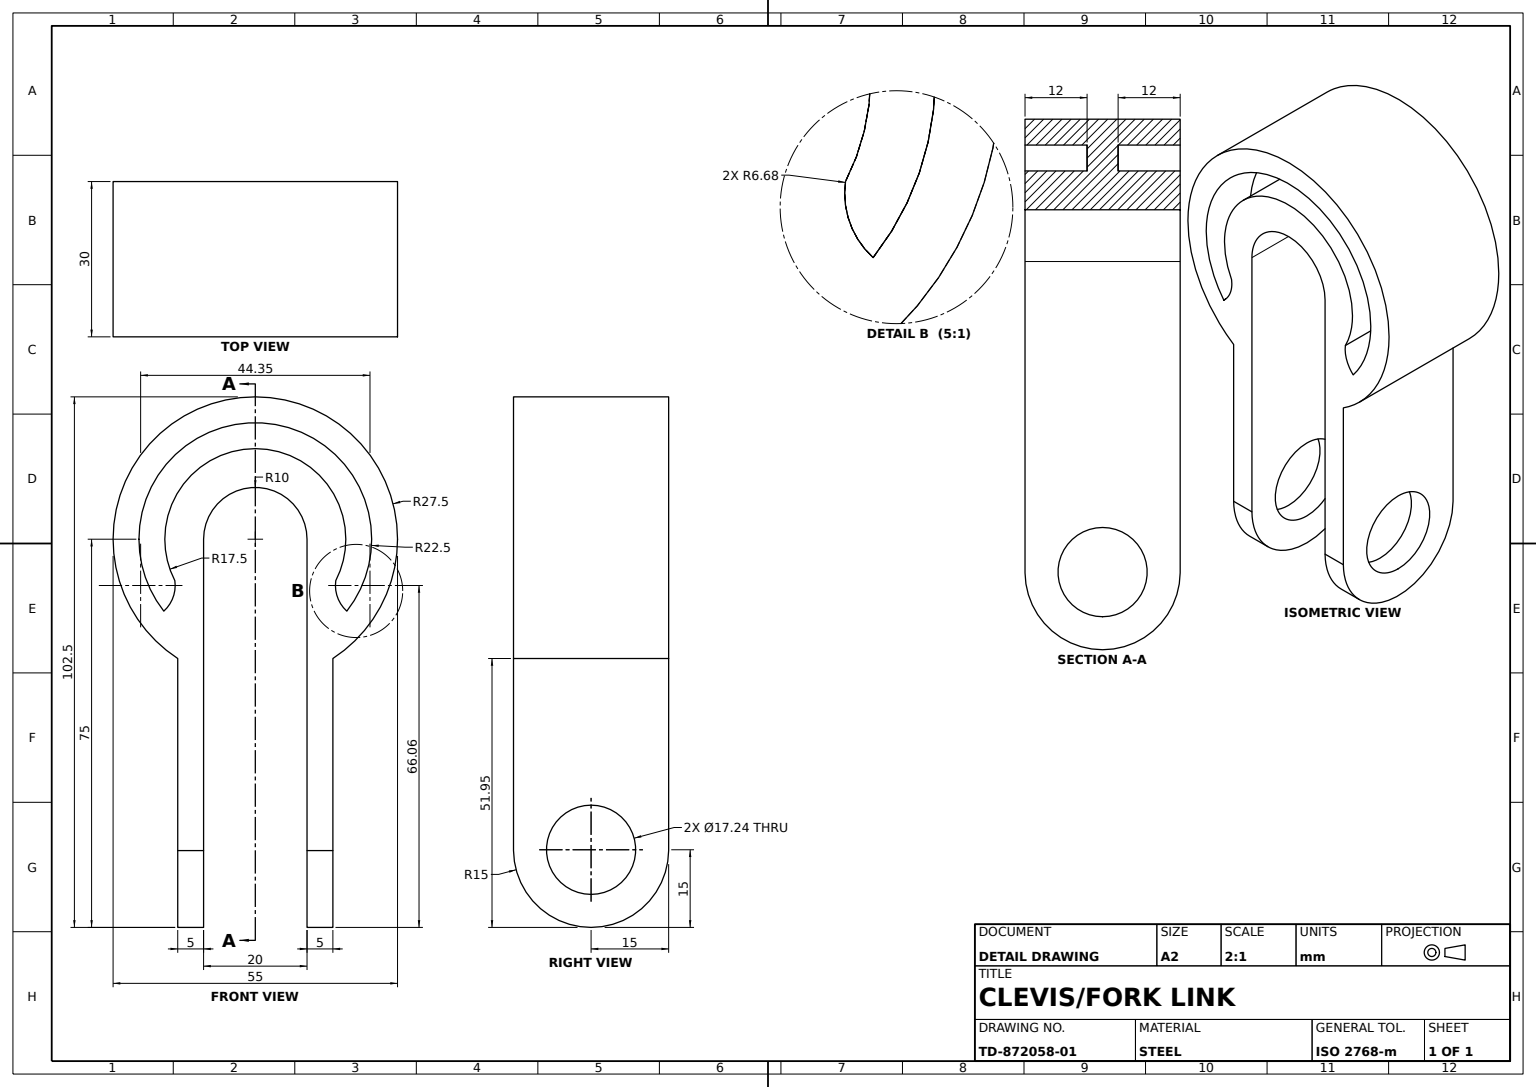
from build123d import *

# Parameters (mm, degrees)
CLEVIS_BODY_DEPTH        = 15
PROFILE_START            = 15
PROFILE_CUT_A_12MM_DEPTH = 12
PROFILE_START_2          = -15
PROFILE_CUT_B_12MM_DEPTH = 12
HEAD_SLOT_SKETCH_R       = 8.62165443
HEAD_SLOT_CUT_DEPTH      = 88.5


with BuildPart() as part:
    # Clevis Profile Sketch → Clevis Body (new, symmetric)
    # profile 1 of 3: a face of its own
    with BuildSketch(Plane.XY):
        with BuildLine():
            ThreePointArc((-15, 0), (0, 15), (15, 0))
            Line((15, 0), (15, -23.048861143))
            ThreePointArc((15, -23.048861143), (0, 27.5), (-15, -23.048861143))
            Line((-15, -23.048861143), (-15, 0))
        make_face()
        with BuildLine():
            ThreePointArc((-17.692907365, -13.900037013), (0, 22.5), (17.692907365, -13.900037013))
            ThreePointArc((17.692907365, -13.900037013), (15.892818017, -11.22254507), (15.557337138, -8.013692106))
            ThreePointArc((15.557337138, -8.013692106), (0, 17.5), (-15.557337138, -8.013692106))
            ThreePointArc((-15.557337138, -8.013692106), (-15.892818017, -11.22254507), (-17.692907365, -13.900037013))
        make_face(mode=Mode.SUBTRACT)
    # profile 2 of 3: a face of its own
    with BuildSketch(Plane.XY):
        with BuildLine():
            ThreePointArc((17.692907365, -13.900037013), (15.892818017, -11.22254507), (15.557337138, -8.013692106))
            ThreePointArc((15.557337138, -8.013692106), (0, 17.5), (-15.557337138, -8.013692106))
            ThreePointArc((-15.557337138, -8.013692106), (-15.892818017, -11.22254507), (-17.692907365, -13.900037013))
            ThreePointArc((-17.692907365, -13.900037013), (0, 22.5), (17.692907365, -13.900037013))
        make_face()
    # profile 3 of 3: a face of its own
    with BuildSketch(Plane.XY):
        with BuildLine():
            ThreePointArc((10, 0), (0, 10), (-10, 0))
            Line((-10, 0), (-10, -75))
            Line((-10, -75), (-15, -75))
            Line((-15, -75), (-15, 0))
            ThreePointArc((-15, 0), (0, 15), (15, 0))
            Line((15, 0), (15, -75))
            Line((15, -75), (10, -75))
            Line((10, -75), (10, 0))
        make_face()
    extrude(amount=CLEVIS_BODY_DEPTH, both=True)

    # Sketch1_3 → Profile Cut A 12mm (cut)
    with BuildSketch(Plane.XY.offset(PROFILE_START)):
        with BuildLine():
            ThreePointArc((17.692907365, -13.900037013), (15.892818017, -11.22254507), (15.557337138, -8.013692106))
            ThreePointArc((15.557337138, -8.013692106), (0, 17.5), (-15.557337138, -8.013692106))
            ThreePointArc((-15.557337138, -8.013692106), (-15.892818017, -11.22254507), (-17.692907365, -13.900037013))
            ThreePointArc((-17.692907365, -13.900037013), (0, 22.5), (17.692907365, -13.900037013))
        make_face()
    extrude(amount=-PROFILE_CUT_A_12MM_DEPTH, mode=Mode.SUBTRACT)

    # Sketch1_4 → Profile Cut B 12mm (cut)
    with BuildSketch(Plane.XY.offset(PROFILE_START_2)):
        with BuildLine():
            ThreePointArc((17.692907365, -13.900037013), (15.892818017, -11.22254507), (15.557337138, -8.013692106))
            ThreePointArc((15.557337138, -8.013692106), (0, 17.5), (-15.557337138, -8.013692106))
            ThreePointArc((-15.557337138, -8.013692106), (-15.892818017, -11.22254507), (-17.692907365, -13.900037013))
            ThreePointArc((-17.692907365, -13.900037013), (0, 22.5), (17.692907365, -13.900037013))
        make_face()
    extrude(amount=PROFILE_CUT_B_12MM_DEPTH, mode=Mode.SUBTRACT)

    # Head Slot Sketch → Head Slot Cut (cut, through all)
    with BuildSketch(Plane(origin=(15, 0, 0), x_dir=(0, 0, -1), z_dir=(1, 0, 0))):
        with Locations(Location((0, -59.999173584, 0), (0, 0, 90))):
            Circle(HEAD_SLOT_SKETCH_R)
        with BuildLine():
            Line((-15, -75), (0, -75))
            ThreePointArc((0, -75), (-10.55136927, -70.661884294), (-15, -60.15663199))
            Line((-15, -60.15663199), (-15, -75))
        make_face()
        with BuildLine():
            Line((15, -75), (15, -60.15663199))
            ThreePointArc((15, -60.15663199), (10.55136927, -70.661884294), (0, -75))
            Line((0, -75), (15, -75))
        make_face()
    extrude(amount=-HEAD_SLOT_CUT_DEPTH, mode=Mode.SUBTRACT)


solid = part.part
